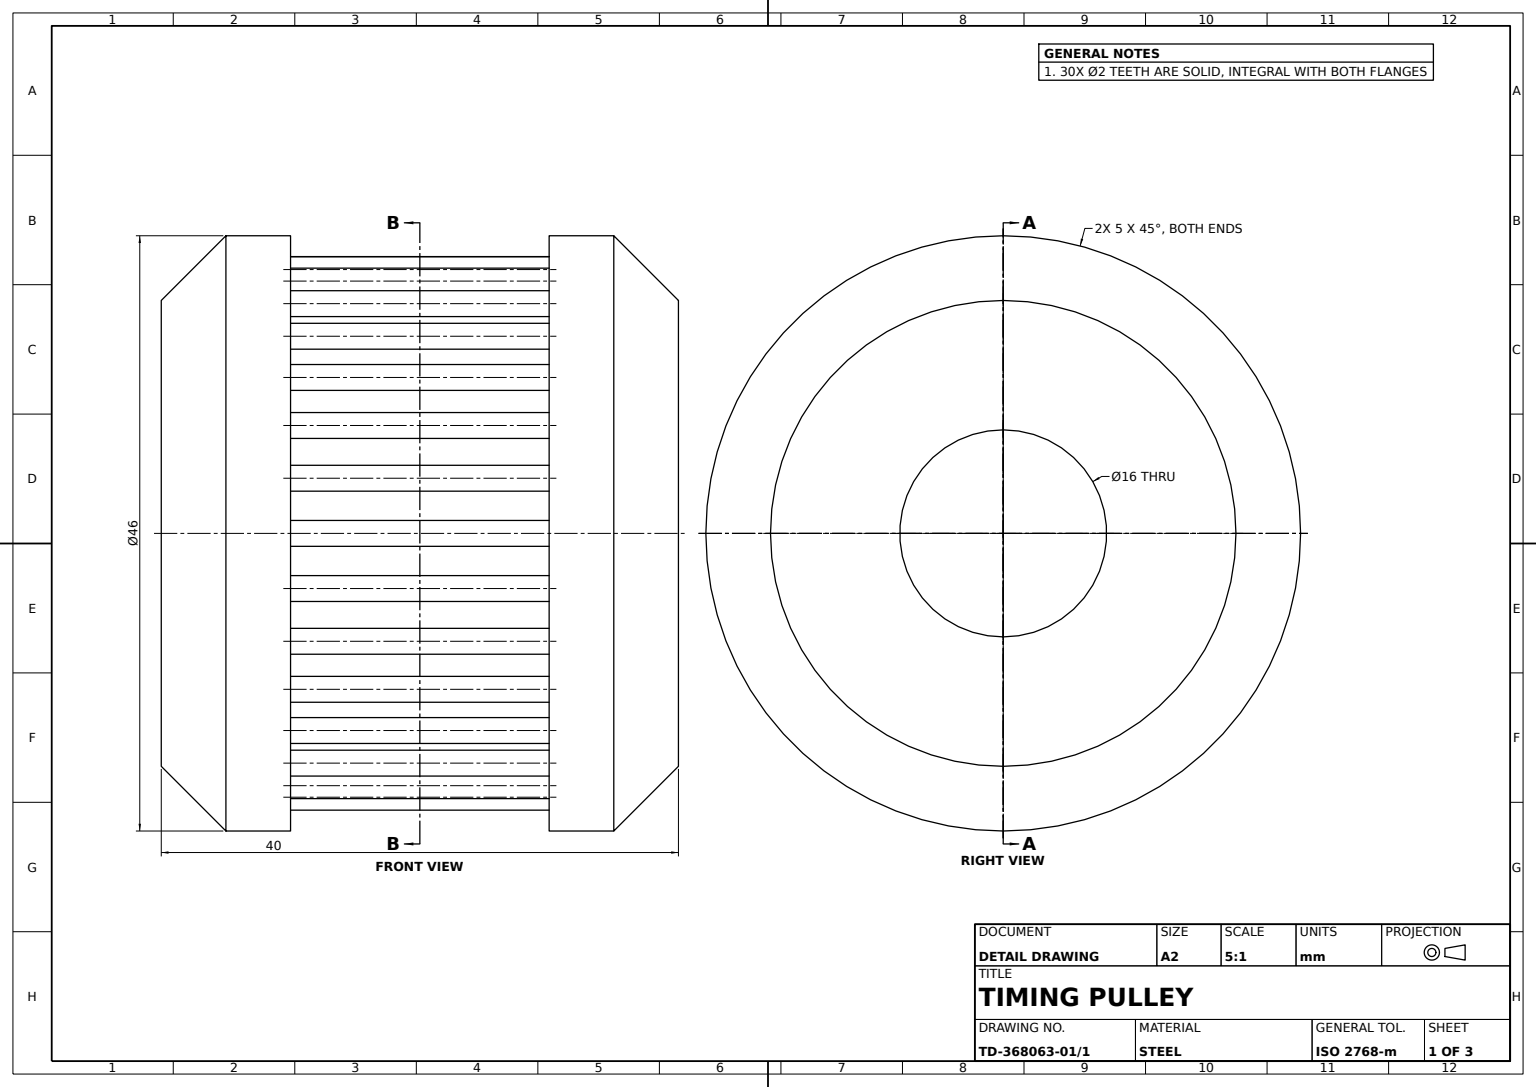
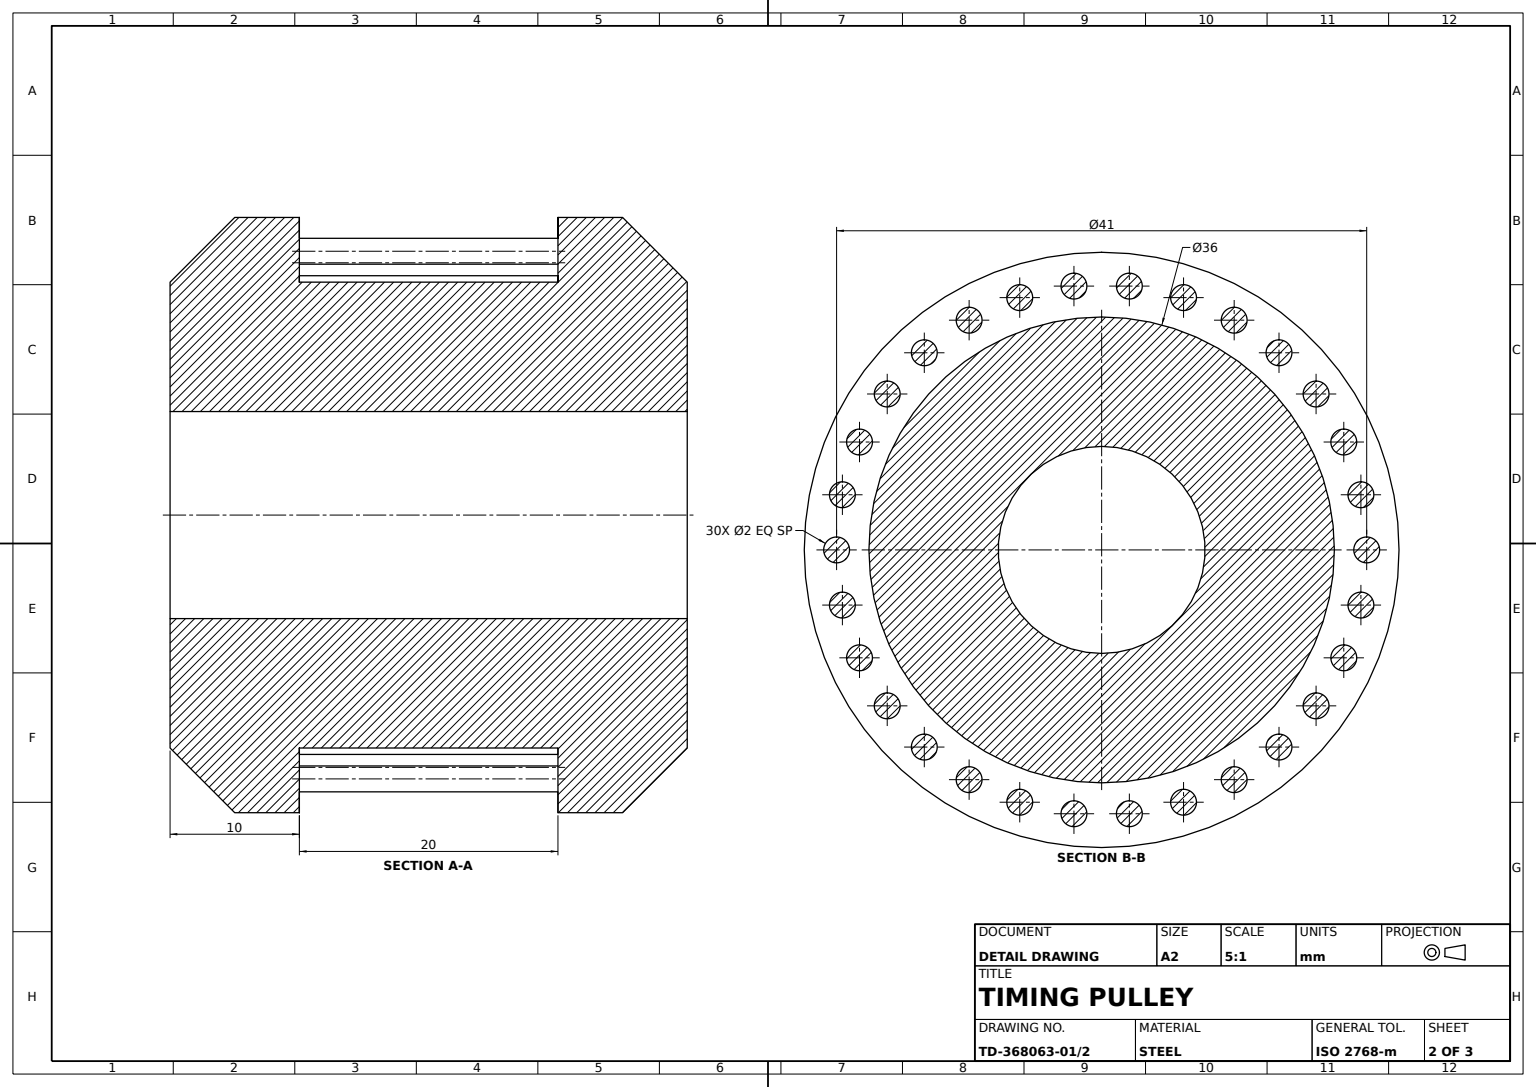
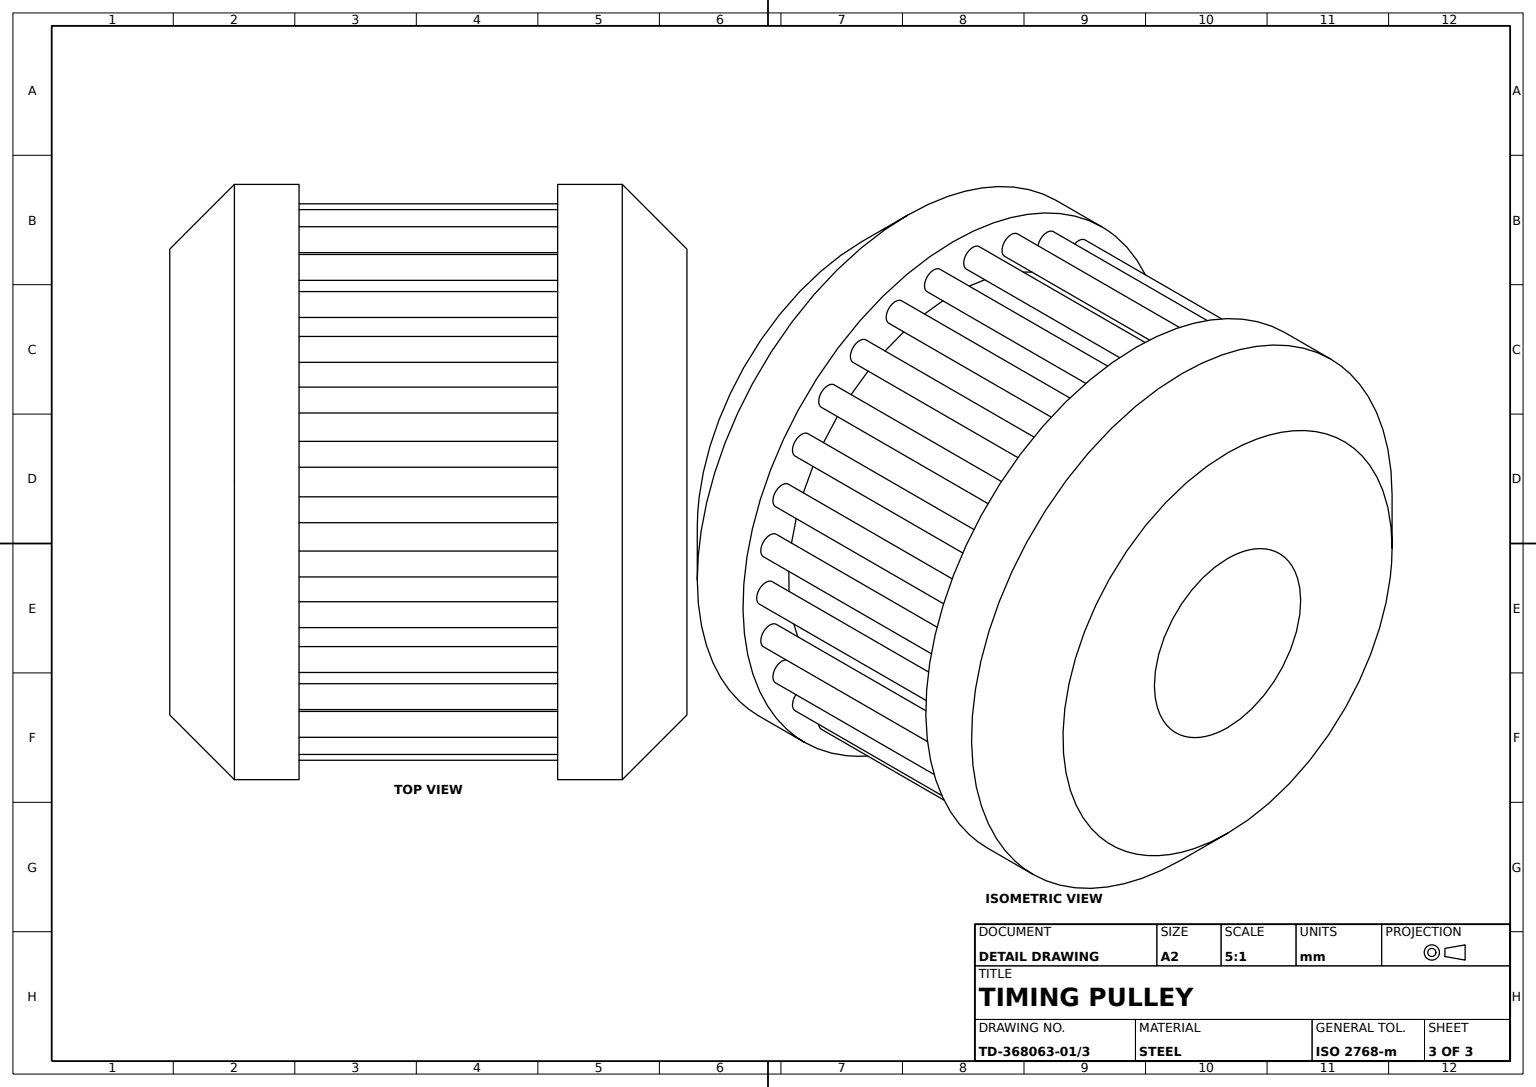
SolidWorks part; units mm, degrees
material "Plain Carbon Steel"
ref_plane "Front Plane" through (0, 0, 0) normal (0, 0, 1) x (1, 0, 0)
ref_plane "Top Plane" through (0, 0, 0) normal (0, 1, 0) x (1, 0, 0)
ref_plane "Right Plane" through (0, 0, 0) normal (1, 0, 0) x (0, 0, -1)
sketch "Pulley Body Profile" plane through (0, 0, 0) normal (0, 0, 1) x (1, 0, 0)
  line L0 (0, 32.6364) -> (0, -35.3636) construction
  line L1 (8, 40) -> (8, 0)
  line L2 (8, 0) -> (18, 0)
  line L3 (23, 5) -> (23, 10)
  line L4 (23, 10) -> (18, 10)
  line L5 (18, 10) -> (18, 30)
  line L6 (18, 30) -> (23, 30)
  line L7 (23, 30) -> (23, 35)
  line L8 (18, 40) -> (8, 40)
  line L9 (18, 0) -> (23, 5)
  line L10 (23, 35) -> (18, 40)
  point P5 (23, 0)
  point P11 (23, 40)
  dimension "D1" = 40
  dimension "D2" = 15
  dimension "D3" = 10
  dimension "D4" = 20
  dimension "D5" = 5
  dimension "D6" = 8
revolve "Pulley Body" add sketch "Pulley Body Profile" angle 360 about L0
sketch "Tooth Profile" plane through (0, 30, 0) normal (0, -1, 0) x (1, 0, 0)
  line L0 (-32.5425, 0) -> (31.6318, -0.3946) construction
  line L1 (0, 37.3281) -> (0, -39.846) construction
  circle A0 centre (0, 20.5) radius 1
  dimension "D2" = 2
  dimension "D1" = 20.5
  dimension "D3" = 32.5425
  dimension "D4" = 31.6318
  dimension "D5" = 0.3946
extrude "Tooth" add sketch "Tooth Profile" along normal blind 20
pattern_circular "Tooth Pattern 30x" count 30 over 360 about axis through (0, 0, 0) along (0, 1, 0) of "Tooth"
